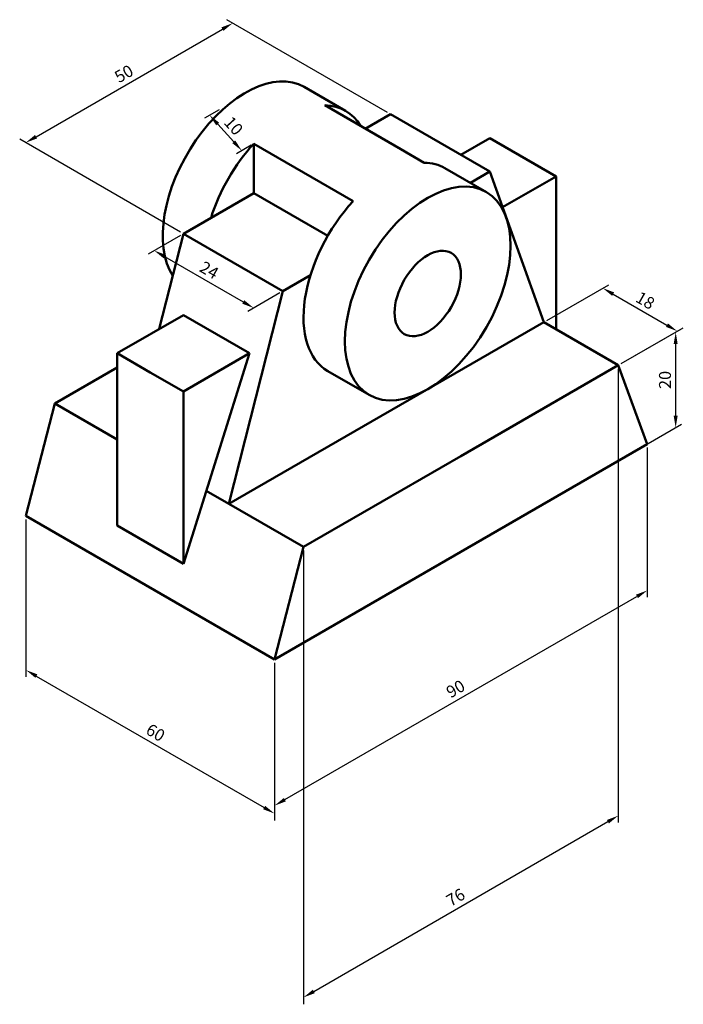
# Model space of a CAD drawing. Units: millimetres. Extents: x 2219 to 2357, y 1646 to 1852.
import ezdxf

# ---------------------------------------------------------------- set-up
doc = ezdxf.new("R2010")
doc.units = ezdxf.units.MM
doc.layers.add('M-DIMS', color=2, linetype='Continuous', lineweight=25)
doc.layers.add('M-OUTL', color=7, linetype='Continuous', lineweight=50)
doc.styles.get("Standard").update_dxf_attribs({"font": 'arial.ttf'})
doc.dimstyles.new('ISO-25', dxfattribs={"dimtxt": 2.5, "dimasz": 2.5, "dimexe": 1.25, "dimexo": 0.625, "dimtad": 1, "dimtxsty": 'Standard', "dimcen": 2.5, "dimadec": 0, "dimazin": 0, "dimtfac": 1, "dimtmove": 0, "dimatfit": 3, "dimfxl": 1, "dimarcsym": 0})

# ---------------------------------------------------------------- blocks, each defined once
blk = doc.blocks.new('*D1')
at = {"layer": 'Defpoints', "color": 0, "transparency": 16777216}
for p in [(2219.89, 1747.78), (2271.85, 1717.78), (2271.85, 1685.54)]:
    blk.add_point(p, dxfattribs=at)
at = {"layer": 'M-DIMS', "color": 0, "lineweight": -2, "transparency": 16777216}
for p, q in [((2219.89, 1747.06), (2219.89, 1714.1)), ((2271.85, 1717.06), (2271.85, 1684.1)), ((2222.05, 1714.29), (2269.69, 1686.79))]:
    blk.add_line(p, q, dxfattribs=at)
at = {"layer": 'M-DIMS', "color": 0, "transparency": 16777216}
for points in [[(2222.26, 1714.65), (2221.85, 1713.93), (2219.89, 1715.54)], [(2269.89, 1687.15), (2269.48, 1686.43), (2271.85, 1685.54)]]:
    blk.add_solid(points, dxfattribs=at)
at = {"layer": 'M-DIMS', "color": 0, "transparency": 16777216, "insert": (2246.82, 1702.19), "char_height": 2.5, "attachment_point": 5, "rotation": 330}
blk.add_mtext('60', dxfattribs=at)
blk = doc.blocks.new('*D2')
at = {"layer": 'Defpoints', "color": 0, "transparency": 16777216}
for p in [(2349.79, 1762.78), (2349.79, 1732.19), (2271.85, 1717.78)]:
    blk.add_point(p, dxfattribs=at)
at = {"layer": 'M-DIMS', "color": 0, "lineweight": -2, "transparency": 16777216}
for p, q in [((2349.79, 1762.06), (2349.79, 1730.75)), ((2274.02, 1688.44), (2347.63, 1730.94)), ((2271.85, 1717.06), (2271.85, 1685.75))]:
    blk.add_line(p, q, dxfattribs=at)
at = {"layer": 'M-DIMS', "color": 0, "transparency": 16777216}
for points in [[(2347.42, 1731.3), (2347.84, 1730.58), (2349.79, 1732.19)], [(2273.81, 1688.8), (2274.22, 1688.08), (2271.85, 1687.19)]]:
    blk.add_solid(points, dxfattribs=at)
at = {"layer": 'M-DIMS', "color": 0, "transparency": 16777216, "insert": (2309.87, 1711.34), "char_height": 2.5, "attachment_point": 5, "rotation": 30}
blk.add_mtext('90', dxfattribs=at)
blk = doc.blocks.new('*D3')
at = {"layer": 'Defpoints', "color": 0, "transparency": 16777216}
for p in [(2263.12, 1850.82), (2296.1, 1831.78), (2252.8, 1806.78)]:
    blk.add_point(p, dxfattribs=at)
at = {"layer": 'M-DIMS', "color": 0, "lineweight": -2, "transparency": 16777216}
for p, q in [((2295.47, 1832.14), (2261.87, 1851.54)), ((2221.99, 1827.07), (2260.96, 1849.57)), ((2252.17, 1807.14), (2218.57, 1826.54))]:
    blk.add_line(p, q, dxfattribs=at)
at = {"layer": 'M-DIMS', "color": 0, "transparency": 16777216}
for points in [[(2260.75, 1849.93), (2261.17, 1849.21), (2263.12, 1850.82)], [(2221.78, 1827.43), (2222.2, 1826.71), (2219.82, 1825.82)]]:
    blk.add_solid(points, dxfattribs=at)
at = {"layer": 'M-DIMS', "color": 0, "transparency": 16777216, "insert": (2240.52, 1839.97), "char_height": 2.5, "attachment_point": 5, "rotation": 30}
blk.add_mtext('50', dxfattribs=at)
blk = doc.blocks.new('*D4')
at = {"layer": 'Defpoints', "color": 0, "transparency": 16777216}
for p in [(2260.8, 1833.02), (2258.29, 1831.57), (2267.52, 1825.61)]:
    blk.add_point(p, dxfattribs=at)
at = {"layer": 'M-DIMS', "color": 0, "lineweight": -2, "transparency": 16777216}
for p, q in [((2260.25, 1832.7), (2257.18, 1830.93)), ((2263.33, 1826.01), (2259.97, 1829.72)), ((2266.97, 1825.29), (2263.9, 1823.52))]:
    blk.add_line(p, q, dxfattribs=at)
at = {"layer": 'M-DIMS', "color": 0, "transparency": 16777216}
for points in [[(2260.28, 1830), (2259.66, 1829.44), (2258.29, 1831.57)], [(2263.64, 1826.29), (2263.02, 1825.73), (2265.01, 1824.16)]]:
    blk.add_solid(points, dxfattribs=at)
at = {"layer": 'M-DIMS', "color": 0, "transparency": 16777216, "insert": (2263.06, 1829.14), "char_height": 2.5, "attachment_point": 5, "rotation": 312.215}
blk.add_mtext('10', dxfattribs=at)
blk = doc.blocks.new('*D5')
at = {"layer": 'Defpoints', "color": 0, "transparency": 16777216}
for p in [(2355.73, 1786.21), (2343.73, 1779.28), (2343.73, 1759.28)]:
    blk.add_point(p, dxfattribs=at)
at = {"layer": 'M-DIMS', "color": 0, "lineweight": -2, "transparency": 16777216}
for p, q in [((2344.36, 1779.64), (2356.98, 1786.93)), ((2355.73, 1768.71), (2355.73, 1783.71)), ((2344.36, 1759.64), (2356.98, 1766.93))]:
    blk.add_line(p, q, dxfattribs=at)
at = {"layer": 'M-DIMS', "color": 0, "transparency": 16777216}
for points in [[(2355.31, 1783.71), (2356.14, 1783.71), (2355.73, 1786.21)], [(2355.31, 1768.71), (2356.14, 1768.71), (2355.73, 1766.21)]]:
    blk.add_solid(points, dxfattribs=at)
at = {"layer": 'M-DIMS', "color": 0, "transparency": 16777216, "insert": (2353.82, 1776.21), "char_height": 2.5, "attachment_point": 5, "rotation": 90}
blk.add_mtext('20', dxfattribs=at)
blk = doc.blocks.new('*D6')
at = {"layer": 'Defpoints', "color": 0, "transparency": 16777216}
for p in [(2343.73, 1779.28), (2277.91, 1741.28), (2343.73, 1685.09)]:
    blk.add_point(p, dxfattribs=at)
at = {"layer": 'M-DIMS', "color": 0, "lineweight": -2, "transparency": 16777216}
for p, q in [((2343.73, 1778.56), (2343.73, 1683.65)), ((2277.91, 1740.56), (2277.91, 1645.65)), ((2280.08, 1648.34), (2341.57, 1683.84))]:
    blk.add_line(p, q, dxfattribs=at)
at = {"layer": 'M-DIMS', "color": 0, "transparency": 16777216}
for points in [[(2341.36, 1684.2), (2341.77, 1683.48), (2343.73, 1685.09)], [(2279.87, 1648.7), (2280.29, 1647.98), (2277.91, 1647.09)]]:
    blk.add_solid(points, dxfattribs=at)
at = {"layer": 'M-DIMS', "color": 0, "transparency": 16777216, "insert": (2309.87, 1667.74), "char_height": 2.5, "attachment_point": 5, "rotation": 30}
blk.add_mtext('76', dxfattribs=at)
blk = doc.blocks.new('*D7')
at = {"layer": 'Defpoints', "color": 0, "transparency": 16777216}
for p in [(2328.14, 1788.28), (2356.07, 1786.41), (2343.73, 1779.28)]:
    blk.add_point(p, dxfattribs=at)
at = {"layer": 'M-DIMS', "color": 0, "lineweight": -2, "transparency": 16777216}
for p, q in [((2328.77, 1788.64), (2341.74, 1796.13)), ((2342.65, 1794.16), (2353.91, 1787.66)), ((2344.36, 1779.64), (2357.32, 1787.13))]:
    blk.add_line(p, q, dxfattribs=at)
at = {"layer": 'M-DIMS', "color": 0, "transparency": 16777216}
for points in [[(2342.86, 1794.52), (2342.44, 1793.8), (2340.49, 1795.41)], [(2354.12, 1788.02), (2353.7, 1787.3), (2356.07, 1786.41)]]:
    blk.add_solid(points, dxfattribs=at)
at = {"layer": 'M-DIMS', "color": 0, "transparency": 16777216, "insert": (2349.23, 1792.56), "char_height": 2.5, "attachment_point": 5, "rotation": 330}
blk.add_mtext('18', dxfattribs=at)
blk = doc.blocks.new('*D8')
at = {"layer": 'Defpoints', "color": 0, "transparency": 16777216}
for p in [(2252.8, 1806.78), (2273.58, 1794.78), (2267.49, 1791.26)]:
    blk.add_point(p, dxfattribs=at)
at = {"layer": 'M-DIMS', "color": 0, "lineweight": -2, "transparency": 16777216}
for p, q in [((2252.17, 1806.42), (2245.45, 1802.54)), ((2248.87, 1802.01), (2265.32, 1792.51)), ((2272.96, 1794.42), (2266.24, 1790.54))]:
    blk.add_line(p, q, dxfattribs=at)
at = {"layer": 'M-DIMS', "color": 0, "transparency": 16777216}
for points in [[(2249.08, 1802.38), (2248.66, 1801.65), (2246.7, 1803.26)], [(2265.53, 1792.88), (2265.12, 1792.15), (2267.49, 1791.26)]]:
    blk.add_solid(points, dxfattribs=at)
at = {"layer": 'M-DIMS', "color": 0, "transparency": 16777216, "insert": (2258.04, 1798.89), "char_height": 2.5, "attachment_point": 5, "rotation": 330}
blk.add_mtext('24', dxfattribs=at)

msp = doc.modelspace()

# ---------------------------------------------------------------- linework, layer by layer
at = {"layer": 'M-OUTL'}
for p, q in [((2278.035, 1837.496), (2286.696, 1832.496)), ((2298.233, 1824.479), (2282.362, 1833.642)), ((2290.84, 1828.746), (2296.099, 1831.782)), ((2290.84, 1828.746), (2296.099, 1831.782)), ((2296.099, 1831.782), (2316.883, 1819.782)), ((2310.821, 1823.282), (2316.883, 1826.782)), ((2316.883, 1826.782), (2330.74, 1818.782)), ((2267.52, 1815.282), (2267.52, 1825.613)), ((2267.52, 1825.613), (2288.305, 1813.613)), ((2298.233, 1824.479), (2303.146, 1821.642)), ((2316.14, 1815.496), (2307.48, 1820.496)), ((2316.883, 1819.782), (2312.799, 1817.425)), ((2316.883, 1819.782), (2328.142, 1788.282)), ((2330.74, 1818.782), (2319.55, 1812.322)), ((2330.74, 1818.782), (2330.74, 1786.782)), ((2252.798, 1806.782), (2267.52, 1815.282)), ((2252.798, 1806.782), (2267.52, 1815.282)), ((2267.52, 1815.282), (2282.985, 1806.353)), ((2252.798, 1806.782), (2247.761, 1786.874)), ((2273.582, 1794.782), (2252.798, 1806.782)), ((2279.358, 1798.117), (2273.582, 1794.782)), ((2273.582, 1794.782), (2262.324, 1750.282)), ((2238.941, 1781.782), (2252.798, 1789.782)), ((2252.798, 1789.782), (2266.654, 1781.782)), ((2262.324, 1750.282), (2328.142, 1788.282)), ((2328.142, 1788.282), (2343.73, 1779.282)), ((2245.869, 1777.782), (2238.941, 1781.782)), ((2238.941, 1781.782), (2238.941, 1745.782)), ((2252.798, 1773.782), (2266.654, 1781.782)), ((2266.654, 1781.782), (2252.798, 1737.782)), ((2310.821, 1760.282), (2343.73, 1779.282)), ((2343.73, 1779.282), (2349.792, 1762.782)), ((2225.951, 1771.282), (2238.941, 1778.782)), ((2245.869, 1777.782), (2252.798, 1773.782)), ((2291.646, 1773.069), (2282.985, 1778.069)), ((2252.798, 1737.782), (2252.798, 1773.782)), ((2219.889, 1747.782), (2225.951, 1771.282)), ((2238.941, 1763.782), (2225.951, 1771.282)), ((2271.85, 1717.782), (2349.792, 1762.782)), ((2310.821, 1760.282), (2277.912, 1741.282)), ((2262.324, 1750.282), (2257.594, 1753.013)), ((2277.912, 1741.282), (2262.324, 1750.282)), ((2219.889, 1747.782), (2271.85, 1717.782)), ((2238.941, 1745.782), (2252.798, 1737.782)), ((2277.912, 1741.282), (2271.85, 1717.782))]:
    msp.add_line(p, q, dxfattribs=at)
for centre, start_param, end_param in [((2265.788, 1816.282), 3.1415927, 5.9949348), ((2274.448, 1811.282), 9.1138686, 9.7356874), ((2274.448, 1811.282), 4.3385077, 5.0862703), ((2295.233, 1799.282), 3.1415927, 3.4525021), ((2295.233, 1799.282), 4.3385077, 6.2831853)]:
    msp.add_ellipse(centre, major_axis=(-12.247, -21.213), ratio=0.5773503, start_param=start_param, end_param=end_param, dxfattribs=at)
for major_axis in [(-12.247, -21.213), (-4.899, -8.485)]:
    msp.add_ellipse((2303.893, 1794.282), major_axis=major_axis, ratio=0.5773503, dxfattribs=at)

# ---------------------------------------------------------------- dimensions: what is measured, and where the dimension line sits
at = {"layer": 'M-DIMS'}
for p1, p2, distance, picture, middle in [((2252.798, 1806.782), (2296.099, 1831.782), 32.975, '*D3', (2240.523, 1839.967)), ((2267.52, 1825.613), (2260.801, 1833.019), 2.837, '*D4', (2263.055, 1829.142)), ((2252.798, 1806.782), (2273.582, 1794.782), -6.093, '*D8', (2258.037, 1798.893)), ((2328.142, 1788.282), (2343.73, 1779.282), 12.344, '*D7', (2349.23, 1792.556)), ((2343.73, 1759.282), (2343.73, 1779.282), -11.996, '*D5', (2353.825, 1776.208)), ((2277.912, 1741.282), (2343.73, 1779.282), -81.574, '*D6', (2309.871, 1667.736)), ((2271.85, 1717.782), (2349.792, 1762.782), -26.494, '*D2', (2309.871, 1711.336)), ((2219.889, 1747.782), (2271.85, 1717.782), -27.92, '*D1', (2246.82, 1702.189))]:
    dim = msp.add_aligned_dim(p1=p1, p2=p2, distance=distance, dimstyle='ISO-25', override={"dimclrd": 0, "dimclre": 0, "dimclrt": 0}, dxfattribs=at)
    dim.commit()
    dim.dimension.update_dxf_attribs({"geometry": picture, "text_midpoint": middle})

doc.saveas('drawing.dxf')
